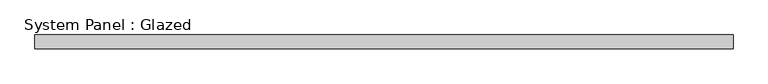
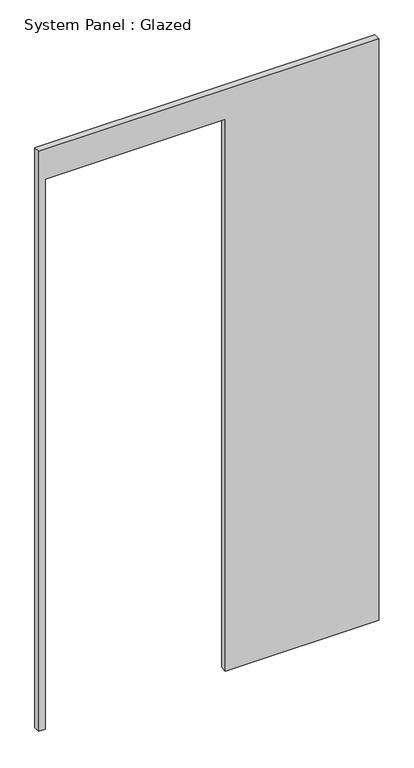
"""IFC4 building model written with IfcOpenShell, lengths in millimetres: plate geometry, System Panel : Glazed."""

from ifc_helpers import new_model, si_unit, frame, origin, place, context, project, spatial, polyline, outline, extrude, source, transform, mapped, element, save


def system_panel_glazed_bef2143c(model_context):
    return source(origin(), model_context, "Body", "SweptSolid", [
        extrude(outline(polyline([(0.0, 63.5), (0.0, 647.7), (2343.15, 647.7), (2343.15, -647.7), (6.4344163, -647.7), (6.4344163, -622.3), (2222.5, -622.3), (2222.5, 63.5), (0.0, 63.5)])), frame((0.0, 19.05, 0.0), z_axis=(0.0, 1.0, 0.0), x_axis=(0.0, 0.0, 1.0)), (0.0, 0.0, 1.0), 25.4),
    ])


if __name__ == "__main__":
    model = new_model("IFC4")
    model_context = context("Model", 3, world=origin())
    ifc_project = project(units=[si_unit("LENGTHUNIT", "METRE", prefix="MILLI")], contexts=[model_context])
    site = spatial("IfcSite", under=ifc_project)
    building = spatial("IfcBuilding", under=site)
    placement = place(None, origin())
    system_panel_glazed_shape = system_panel_glazed_bef2143c(model_context)
    element("IfcPlate", 1, ObjectType="System Panel : Glazed", at=placement, inside=building, context=model_context, shape_type="MappedRepresentation", body=[
        mapped(system_panel_glazed_shape, transform((0.0, 0.0, 0.0), x_axis=(1.0, 0.0, 0.0), y_axis=(0.0, 1.0, 0.0), z_axis=(0.0, 0.0, 1.0))),
    ])
    save(model, "model.ifc")

# Revit data of these elements
# Type "System Panel : Glazed"
#   Construction Type Id = "GSP4R"
#   Analytic Construction = "1/8 in Pilkington single glazing"
#   Visual Light Transmittance = 0.9
#   Solar Heat Gain Coefficient = 0.86
#   Heat Transfer Coefficient (U) = 1.18115 BTU/(h·ft²·°F)
# Element 1 (IfcPlate, "System Panel : Glazed")
#   Materials on its faces: "Glass"
# Materials
#   "Glass": class "Glass", colour RGB 0 128 192, transparency 0.75, Description = "Soda Lime Glass", Cost = 0
